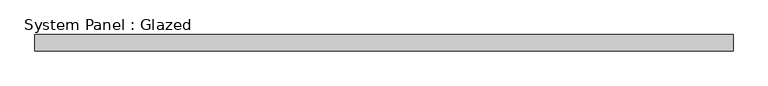
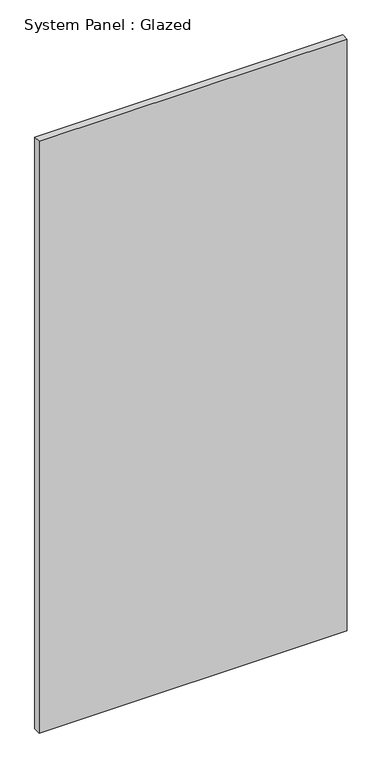
"""IFC4 building model written with IfcOpenShell, lengths in millimetres: plate geometry, System Panel : Glazed."""

from ifc_helpers import new_model, si_unit, origin, origin_with_axes, place, context, project, spatial, polyline, outline, extrude, source, transform, mapped, element, save


def system_panel_glazed_98578528(model_context):
    return source(origin(), model_context, "Body", "SweptSolid", [
        extrude(outline(polyline([(539.75, 19.05), (-539.75, 19.05), (-539.75, 44.45), (539.75, 44.45), (539.75, 19.05)])), origin_with_axes(), (0.0, 0.0, 1.0), 2190.75),
    ])


if __name__ == "__main__":
    model = new_model("IFC4")
    model_context = context("Model", 3, world=origin())
    ifc_project = project(units=[si_unit("LENGTHUNIT", "METRE", prefix="MILLI")], contexts=[model_context])
    site = spatial("IfcSite", under=ifc_project)
    building = spatial("IfcBuilding", under=site)
    placement = place(None, origin())
    system_panel_glazed_shape = system_panel_glazed_98578528(model_context)
    element("IfcPlate", 1, ObjectType="System Panel : Glazed", at=placement, inside=building, context=model_context, shape_type="MappedRepresentation", body=[
        mapped(system_panel_glazed_shape, transform((0.0, 0.0, 0.0), x_axis=(1.0, 0.0, 0.0), y_axis=(0.0, 1.0, 0.0), z_axis=(0.0, 0.0, 1.0))),
    ])
    save(model, "model.ifc")

# Revit data of these elements
# Type "System Panel : Glazed"
#   Construction Type Id = "GSP4R"
#   Analytic Construction = "1/8 in Pilkington single glazing"
#   Visual Light Transmittance = 0.9
#   Solar Heat Gain Coefficient = 0.86
#   Heat Transfer Coefficient (U) = 1.18115 BTU/(h·ft²·°F)
#   Define Thermal Properties by = 1
# Element 1 (IfcPlate, "System Panel : Glazed")
#   Materials on its faces: "Glass"
# Materials
#   "Glass": class "Glass", colour RGB 0 128 192, transparency 0.75, Description = "Soda Lime Glass", Cost = 0
